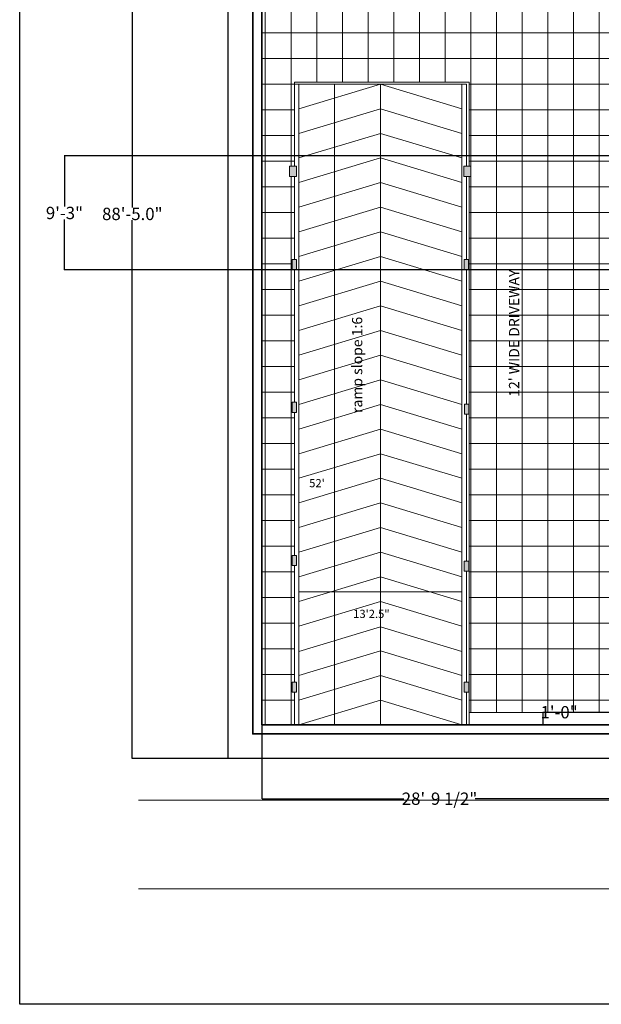
# Model space of a CAD drawing. Units: inches. Extents: x 48986 to 50522, y 132527 to 134098.
# Tile 1 of 4: x 48986 to 49552, y 132529 to 133488. Entities that reach past the tile are written whole.
import ezdxf

# ---------------------------------------------------------------- set-up
doc = ezdxf.new("R2010")
doc.units = ezdxf.units.IN
doc.header["$MEASUREMENT"] = 0
for name, color, linetype, lineweight in [('A-ANNO-DIMS', 2, 'Continuous', 18), ('A-ANNO-TEXT', 7, 'Continuous', 18), ('A-ANNO-TTLB', 7, 'Continuous', 25), ('A-FLOR-PATT', 94, 'Continuous', 9), ('A-FLOR-PKNG', 140, 'Continuous', 18), ('A-FLOR-RAMP', 7, 'Continuous', 18), ('A-RAMP-PATT', 215, 'Continuous', 13), ('C-PROP', 160, 'Continuous', 25), ('C-ROAD', 7, 'Continuous', 18), ('WALLS', 140, 'Continuous', 35)]:
    doc.layers.add(name, color=color, linetype=linetype, lineweight=lineweight)
doc.styles.get("Standard").update_dxf_attribs({"font": 'arial.ttf'})
doc.dimstyles.get("Standard").update_dxf_attribs({"dimtxt": 12, "dimasz": 0.18, "dimexe": 0.18, "dimexo": 0.0625, "dimgap": 0.09, "dimtad": 0, "dimtih": 1, "dimtoh": 1, "dimdec": 1, "dimzin": 0, "dimdsep": 46, "dimlunit": 3, "dimtxsty": 'Standard', "dimcen": 0.09, "dimadec": 0, "dimazin": 0, "dimtfac": 1, "dimtdec": 1, "dimtofl": 0, "dimtmove": 0, "dimatfit": 3, "dimfxl": 1, "dimtolj": 1, "dimtzin": 0, "dimarcsym": 0})

# ---------------------------------------------------------------- blocks, each defined once
blk = doc.blocks.new('*D3')
at = {"layer": 'A-ANNO-DIMS', "color": 0, "lineweight": -2, "transparency": 16777216}
for p, q in [((49188.73, 133829.06), (49095.4, 133829.06)), ((49095.58, 133828.88), (49095.58, 133304.77)), ((49095.58, 132768.24), (49095.58, 133292.34)), ((49188.73, 132768.06), (49095.4, 132768.06))]:
    blk.add_line(p, q, dxfattribs=at)
at = {"layer": 'A-ANNO-DIMS', "color": 0, "transparency": 16777216}
for points in [[(49095.55, 133828.88), (49095.61, 133828.88), (49095.58, 133829.06)], [(49095.55, 132768.24), (49095.61, 132768.24), (49095.58, 132768.06)]]:
    blk.add_solid(points, dxfattribs=at)
at = {"layer": 'Defpoints', "color": 0, "transparency": 16777216}
for p in [(49188.79, 133829.06), (49095.58, 132768.06), (49188.79, 132768.06)]:
    blk.add_point(p, dxfattribs=at)
at = {"layer": 'A-ANNO-DIMS', "color": 0, "transparency": 16777216, "insert": (49095.58, 133298.56), "char_height": 12, "attachment_point": 5}
blk.add_mtext('\\A1;88\'-5.0"', dxfattribs=at)
blk = doc.blocks.new('*D27')
at = {"layer": 'A-ANNO-DIMS', "color": 0, "lineweight": -2, "transparency": 16777216}
for p, q in [((49221.79, 132800.99), (49221.79, 132728.83)), ((49567.36, 132800.99), (49567.36, 132728.83)), ((49221.97, 132729.01), (49359.79, 132729.01)), ((49567.18, 132729.01), (49429.36, 132729.01))]:
    blk.add_line(p, q, dxfattribs=at)
at = {"layer": 'A-ANNO-DIMS', "color": 0, "transparency": 16777216}
for points in [[(49221.97, 132729.04), (49221.97, 132728.98), (49221.79, 132729.01)], [(49567.18, 132729.04), (49567.18, 132728.98), (49567.36, 132729.01)]]:
    blk.add_solid(points, dxfattribs=at)
at = {"layer": 'Defpoints', "color": 0, "transparency": 16777216}
for p in [(49221.79, 132801.06), (49567.36, 132801.06), (49221.79, 132729.01)]:
    blk.add_point(p, dxfattribs=at)
at = {"layer": 'A-ANNO-DIMS', "color": 0, "transparency": 16777216, "insert": (49394.57, 132729.01), "char_height": 12, "attachment_point": 5}
blk.add_mtext('\\A1;28\'-9 1/2"', dxfattribs=at)
blk = doc.blocks.new('*D30')
at = {"layer": 'A-ANNO-DIMS', "color": 0, "lineweight": -2, "transparency": 16777216}
for p, q in [((50139.82, 133355.06), (49029.36, 133355.06)), ((49029.54, 133354.88), (49029.54, 133305.73)), ((49029.54, 133244.15), (49029.54, 133293.29)), ((50139.82, 133243.97), (49029.36, 133243.97))]:
    blk.add_line(p, q, dxfattribs=at)
at = {"layer": 'A-ANNO-DIMS', "color": 0, "transparency": 16777216}
for points in [[(49029.51, 133354.88), (49029.57, 133354.88), (49029.54, 133355.06)], [(49029.51, 133244.15), (49029.57, 133244.15), (49029.54, 133243.97)]]:
    blk.add_solid(points, dxfattribs=at)
at = {"layer": 'Defpoints', "color": 0, "transparency": 16777216}
for p in [(49029.54, 133355.06), (50139.88, 133355.06), (50139.88, 133243.97)]:
    blk.add_point(p, dxfattribs=at)
at = {"layer": 'A-ANNO-DIMS', "color": 0, "transparency": 16777216, "insert": (49029.54, 133299.51), "char_height": 12, "attachment_point": 5}
blk.add_mtext('\\A1;9\'-3"', dxfattribs=at)
blk = doc.blocks.new('*D45')
at = {"layer": 'A-ANNO-DIMS', "color": 0, "lineweight": -2, "transparency": 16777216}
for p, q in [((49567.3, 132813.06), (49495.13, 132813.06)), ((49495.31, 132813.06), (49495.31, 132813.24)), ((49495.31, 132813.24), (49495.49, 132813.24)), ((49495.31, 132801.24), (49495.31, 132812.88)), ((49567.3, 132801.06), (49495.13, 132801.06))]:
    blk.add_line(p, q, dxfattribs=at)
at = {"layer": 'A-ANNO-DIMS', "color": 0, "transparency": 16777216}
for points in [[(49495.28, 132812.88), (49495.34, 132812.88), (49495.31, 132813.06)], [(49495.28, 132801.24), (49495.34, 132801.24), (49495.31, 132801.06)]]:
    blk.add_solid(points, dxfattribs=at)
at = {"layer": 'Defpoints', "color": 0, "transparency": 16777216}
for p in [(49495.31, 132813.06), (49567.36, 132813.06), (49567.36, 132801.06)]:
    blk.add_point(p, dxfattribs=at)
at = {"layer": 'A-ANNO-DIMS', "color": 0, "transparency": 16777216, "insert": (49510.96, 132813.24), "char_height": 12, "attachment_point": 5}
blk.add_mtext('\\A1;1\'-0"', dxfattribs=at)

msp = doc.modelspace()

# ---------------------------------------------------------------- hatches: boundary and pattern name
at = {"layer": 'A-FLOR-PATT'}
h = msp.add_hatch(dxfattribs=at)
h.set_pattern_fill('NET', color=256, scale=200)
h.paths.add_polyline_path([(50323.33, 133597.94), (50298.79, 133598.06), (50199.79, 133598.06), (49957.56, 133598.06), (49597.63, 133598.06), (49221.79, 133598.06), (49221.79, 132801.06), (49253.29, 132801.06), (49253.29, 132832.63), (49251.14, 132832.63), (49251.14, 132842.53), (49253.29, 132842.53), (49253.29, 132956.08), (49251.14, 132956.08), (49251.14, 132965.97), (49253.29, 132965.97), (49253.29, 133105.3), (49251.14, 133105.3), (49251.14, 133115.2), (49253.29, 133115.2), (49253.29, 133143.75), (49253.29, 133153.65), (49253.29, 133244.43), (49251.14, 133244.43), (49251.14, 133254.33), (49253.29, 133254.33), (49253.29, 133283.54), (49253.29, 133293.44), (49253.29, 133335.08), (49251.14, 133335.08), (49248.66, 133335.08), (49248.66, 133344.97), (49251.14, 133344.97), (49253.29, 133344.97), (49253.29, 133387.65), (49253.29, 133397.55), (49253.29, 133425.06), (49253.29, 133426.99), (49420.79, 133426.99), (49423.36, 133426.99), (49423.36, 133344.97), (49425.09, 133344.97), (49425.09, 133335.08), (49423.36, 133335.08), (49423.36, 132813.06), (49567.36, 132813.06), (49567.36, 133229.31), (49567.36, 133241.64), (49567.36, 133265.64), (49567.36, 133335.08), (49567.36, 133344.97), (49567.36, 133361.98), (49567.36, 133385.98), (49567.36, 133426.99), (49591.36, 133426.99), (49690.36, 133426.99), (49817.62, 133426.99), (49817.62, 133427.11), (49841.62, 133427.11), (49995.88, 133426.99), (49995.88, 132801.06), (50139.88, 132801.06), (50139.88, 133259.08, -0.361241), (50136.6, 133263.03, -0.361241), (50139.88, 133266.99), (50139.88, 133448.06), (50303.12, 133448.06), (50303.12, 133472.06), (50323.33, 133472.06)])
at = {"layer": 'A-RAMP-PATT'}
h = msp.add_hatch(color=256, dxfattribs=at)
h.dxf.hatch_style = 1
h.paths.add_polyline_path([(49255.4, 132842.53), (49251.14, 132842.53), (49251.14, 132832.63), (49255.4, 132832.63)])
h.paths.add_polyline_path([(49255.4, 132965.97), (49251.14, 132965.97), (49251.14, 132956.08), (49255.4, 132956.08)])
h.paths.add_polyline_path([(49255.4, 133115.2), (49251.14, 133115.2), (49251.14, 133105.3), (49255.4, 133105.3)])
h.paths.add_polyline_path([(49255.4, 133254.33), (49251.14, 133254.33), (49251.14, 133244.43), (49255.4, 133244.43)])
h.paths.add_polyline_path([(49255.4, 133344.97), (49251.14, 133344.97), (49248.66, 133344.97), (49248.66, 133335.08), (49251.14, 133335.08), (49255.4, 133335.08)])
h.paths.add_polyline_path([(49425.09, 133344.97), (49420.84, 133344.97), (49418.36, 133344.97), (49418.36, 133335.08), (49420.84, 133335.08), (49425.09, 133335.08)])
h.paths.add_polyline_path([(49422.83, 133254.33), (49418.58, 133254.33), (49418.58, 133244.43), (49422.83, 133244.43)])
h.paths.add_polyline_path([(49423.04, 133113.43), (49418.79, 133113.43), (49418.79, 133103.53), (49423.04, 133103.53)])
h.paths.add_polyline_path([(49422.94, 132960.5), (49418.69, 132960.5), (49418.69, 132950.61), (49422.94, 132950.61)])
h.paths.add_polyline_path([(49422.93, 132842.59), (49418.68, 132842.59), (49418.68, 132832.69), (49422.93, 132832.69)])

# ---------------------------------------------------------------- linework, layer by layer
at = {"layer": 'A-ANNO-DIMS'}
for p, q in [((49292.3, 133425.06), (49292.3, 132801.06)), ((49257.79, 132930.53), (49416.29, 132930.53))]:
    msp.add_line(p, q, dxfattribs=at)
at = {"layer": 'A-ANNO-TTLB'}
msp.add_lwpolyline([(48985.99, 134098.01), (50521.96, 134098.01), (50521.96, 132528.75), (48985.99, 132528.75)], close=True, dxfattribs=at)
at = {"layer": 'A-FLOR-PKNG'}
msp.add_lwpolyline([(49567.36, 132837.06), (49567.36, 132801.06), (49567.36, 132813.06), (49423.36, 132813.06)], dxfattribs=at)
at = {"layer": 'A-FLOR-RAMP'}
for p, q in [((49420.79, 133425.06), (49420.79, 133344.97)), ((49420.79, 133335.08), (49420.79, 133254.33)), ((49423.36, 133335.08), (49423.36, 132801.06)), ((49420.79, 133244.43), (49420.79, 133113.43)), ((49253.29, 132965.97), (49253.29, 133105.3)), ((49420.79, 133103.53), (49420.79, 132960.5)), ((49253.29, 132842.53), (49253.29, 132956.08)), ((49420.79, 132950.61), (49420.79, 132842.59)), ((49420.79, 132832.69), (49420.79, 132801.06))]:
    msp.add_line(p, q, dxfattribs=at)
for points in [[(49257.79, 133425.06), (49257.79, 132801.06), (49337.04, 132825.06), (49416.29, 132801.06), (49416.29, 133425.06), (49257.79, 133425.06), (49253.29, 133425.06), (49420.79, 133425.06), (49253.29, 133425.06), (49253.29, 133426.99), (49423.36, 133426.99), (49423.36, 133344.97)], [(49253.29, 133426.99), (49420.79, 133426.99), (49423.36, 133426.99)], [(49253.29, 133425.06), (49253.29, 133397.55), (49253.29, 133387.65), (49253.29, 133344.97)], [(49416.29, 133401.06), (49337.04, 133425.06), (49257.79, 133401.06)], [(49337.04, 133425.06), (49337.04, 132801.06), (49337.04, 132825.06)], [(49416.29, 133377.06), (49337.04, 133401.06), (49257.79, 133377.06)], [(49416.29, 133353.06), (49337.04, 133377.06), (49257.79, 133353.06)], [(49416.29, 133329.06), (49337.04, 133353.06), (49257.79, 133329.06)], [(49253.29, 133335.08), (49253.29, 133293.44), (49253.29, 133283.54), (49253.29, 133254.33)], [(49416.29, 133305.06), (49337.04, 133329.06), (49257.79, 133305.06)], [(49416.29, 133281.06), (49337.04, 133305.06), (49257.79, 133281.06)], [(49416.29, 133257.06), (49337.04, 133281.06), (49257.79, 133257.06)], [(49416.29, 133233.06), (49337.04, 133257.06), (49257.79, 133233.06)], [(49253.29, 133244.43), (49253.29, 133153.65), (49253.29, 133143.75), (49253.29, 133115.2)], [(49416.29, 133209.06), (49337.04, 133233.06), (49257.79, 133209.06)], [(49416.29, 133185.06), (49337.04, 133209.06), (49257.79, 133185.06)], [(49416.29, 133161.06), (49337.04, 133185.06), (49257.79, 133161.06)], [(49416.29, 133137.06), (49337.04, 133161.06), (49257.79, 133137.06)], [(49416.29, 133113.06), (49337.04, 133137.06), (49257.79, 133113.06)], [(49416.29, 133089.06), (49337.04, 133113.06), (49257.79, 133089.06)], [(49416.29, 133065.06), (49337.04, 133089.06), (49257.79, 133065.06)], [(49416.29, 133041.06), (49337.04, 133065.06), (49257.79, 133041.06)], [(49416.29, 133017.06), (49337.04, 133041.06), (49257.79, 133017.06)], [(49416.29, 132993.06), (49337.04, 133017.06), (49257.79, 132993.06)], [(49416.29, 132969.06), (49337.04, 132993.06), (49257.79, 132969.06)], [(49416.29, 132945.06), (49337.04, 132969.06), (49257.79, 132945.06)], [(49416.29, 132921.06), (49337.04, 132945.06), (49257.79, 132921.06)], [(49416.29, 132897.06), (49337.04, 132921.06), (49257.79, 132897.06)], [(49416.29, 132872.49), (49337.04, 132896.49), (49257.79, 132872.49)], [(49416.29, 132849.06), (49337.04, 132873.06), (49257.79, 132849.06)], [(49221.79, 132801.06), (49253.29, 132801.06), (49253.29, 132832.63)]]:
    msp.add_lwpolyline(points, dxfattribs=at)
for points in [[(49255.4, 133335.08), (49255.4, 133344.97), (49251.14, 133344.97), (49248.66, 133344.97), (49248.66, 133335.08), (49251.14, 133335.08)], [(49425.09, 133335.08), (49425.09, 133344.97), (49420.84, 133344.97), (49418.36, 133344.97), (49418.36, 133335.08), (49420.84, 133335.08)], [(49251.14, 133254.33), (49251.14, 133244.43), (49255.4, 133244.43), (49255.4, 133254.33)], [(49418.58, 133254.33), (49418.58, 133244.43), (49422.83, 133244.43), (49422.83, 133254.33)], [(49251.14, 133115.2), (49251.14, 133105.3), (49255.4, 133105.3), (49255.4, 133115.2)], [(49418.79, 133113.43), (49418.79, 133103.53), (49423.04, 133103.53), (49423.04, 133113.43)], [(49251.14, 132965.97), (49251.14, 132956.08), (49255.4, 132956.08), (49255.4, 132965.97)], [(49418.69, 132960.5), (49418.69, 132950.61), (49422.94, 132950.61), (49422.94, 132960.5)], [(49416.29, 132825.06), (49337.04, 132849.06), (49257.79, 132825.06), (49337.04, 132849.06)], [(49251.14, 132842.53), (49251.14, 132832.63), (49255.4, 132832.63), (49255.4, 132842.53)], [(49418.68, 132842.59), (49418.68, 132832.69), (49422.93, 132832.69), (49422.93, 132842.59)]]:
    msp.add_lwpolyline(points, close=True, dxfattribs=at)
at = {"layer": 'C-PROP'}
msp.add_lwpolyline([(49188.79, 133829.06), (50375.29, 133829.06), (50375.29, 132768.06), (49188.79, 132768.06)], close=True, dxfattribs=at)
at = {"layer": 'C-ROAD'}
for p, q in [((49101.59, 132727.74), (50406.89, 132727.74)), ((49101.59, 132641.08), (50406.89, 132641.08))]:
    msp.add_line(p, q, dxfattribs=at)
at = {"layer": 'WALLS'}
msp.add_lwpolyline([(49212.79, 133805.06), (50351.29, 133805.06), (50351.29, 132792.06), (49212.79, 132792.06)], close=True, dxfattribs=at)
msp.add_lwpolyline([(50342.29, 133796.06), (50342.29, 132801.06), (49221.79, 132801.06), (49221.79, 133796.06), (50342.29, 133796.06), (50298.79, 133796.06), (50298.79, 133598.06), (50298.79, 133796.06), (50199.79, 133796.06), (50199.79, 133598.06), (50298.79, 133598.06), (49957.56, 133598.06), (49597.63, 133598.06), (49597.63, 133796.06), (49696.63, 133796.06), (49696.63, 133598.06), (49597.63, 133598.06), (49221.79, 133598.06), (49221.79, 133426.99)], dxfattribs=at)

# ---------------------------------------------------------------- texts
at = {"layer": 'A-ANNO-DIMS', "char_height": 8, "attachment_point": 1}
for s, width, insert in [("52' ", 17.8021, (49267.72, 133040.36)), ('13\'2.5"', 61.4647, (49310.52, 132913.02))]:
    msp.add_mtext_dynamic_manual_height_columns(s, width=width, gutter_width=1, heights=[0], dxfattribs=dict(at, insert=insert))
at = {"layer": 'A-ANNO-TEXT', "char_height": 10, "attachment_point": 1, "rotation": 90}
for s, width, insert in [("12' WIDE DRIVEWAY", 548.8474, (49462.14, 133120.47)), ('ramp slope 1:6', 104.4586, (49309.39, 133104.68))]:
    msp.add_mtext_dynamic_manual_height_columns(s, width=width, gutter_width=1, heights=[0], dxfattribs=dict(at, insert=insert))
at = {"layer": 'A-ANNO-TTLB', "insert": (49459.26, 132582.59), "char_height": 0.2, "attachment_point": 1}
msp.add_mtext_dynamic_manual_height_columns('CELL', width=767.4167, gutter_width=1, heights=[0], dxfattribs=at)

# ---------------------------------------------------------------- dimensions: what is measured, and where the dimension line sits
at = {"layer": 'A-ANNO-DIMS'}
for base, p1, p2, angle, override, picture, middle in [((49095.58, 132768.06), (49188.79, 133829.06), (49188.79, 132768.06), 90, {"dimclrd": 0, "dimclre": 0, "dimclrt": 0}, '*D3', (49095.58, 133298.56)), ((49029.54, 133355.06), (50139.88, 133243.97), (50139.88, 133355.06), 90, {"dimdec": 1, "dimlfac": 1, "dimrnd": 0, "dimzin": 1, "dimdsep": 46, "dimlunit": 4, "dimfrac": 2}, '*D30', (49029.54, 133299.51)), ((49495.31, 132813.06), (49567.36, 132801.06), (49567.36, 132813.06), 90, {"dimdec": 1, "dimlfac": 1, "dimrnd": 0, "dimzin": 1, "dimdsep": 46, "dimlunit": 4, "dimfrac": 2}, '*D45', (49510.96, 132813.24)), ((49221.79, 132729.01), (49567.36, 132801.06), (49221.79, 132801.06), 180, {"dimdec": 1, "dimlfac": 1, "dimrnd": 0, "dimzin": 1, "dimdsep": 46, "dimlunit": 4, "dimfrac": 2}, '*D27', (49394.57, 132729.01))]:
    dim = msp.add_linear_dim(base=base, p1=p1, p2=p2, angle=angle, dimstyle='Standard', override=override, dxfattribs=at)
    dim.commit()
    dim.dimension.update_dxf_attribs({"geometry": picture, "text_midpoint": middle})

doc.saveas('drawing.dxf')
